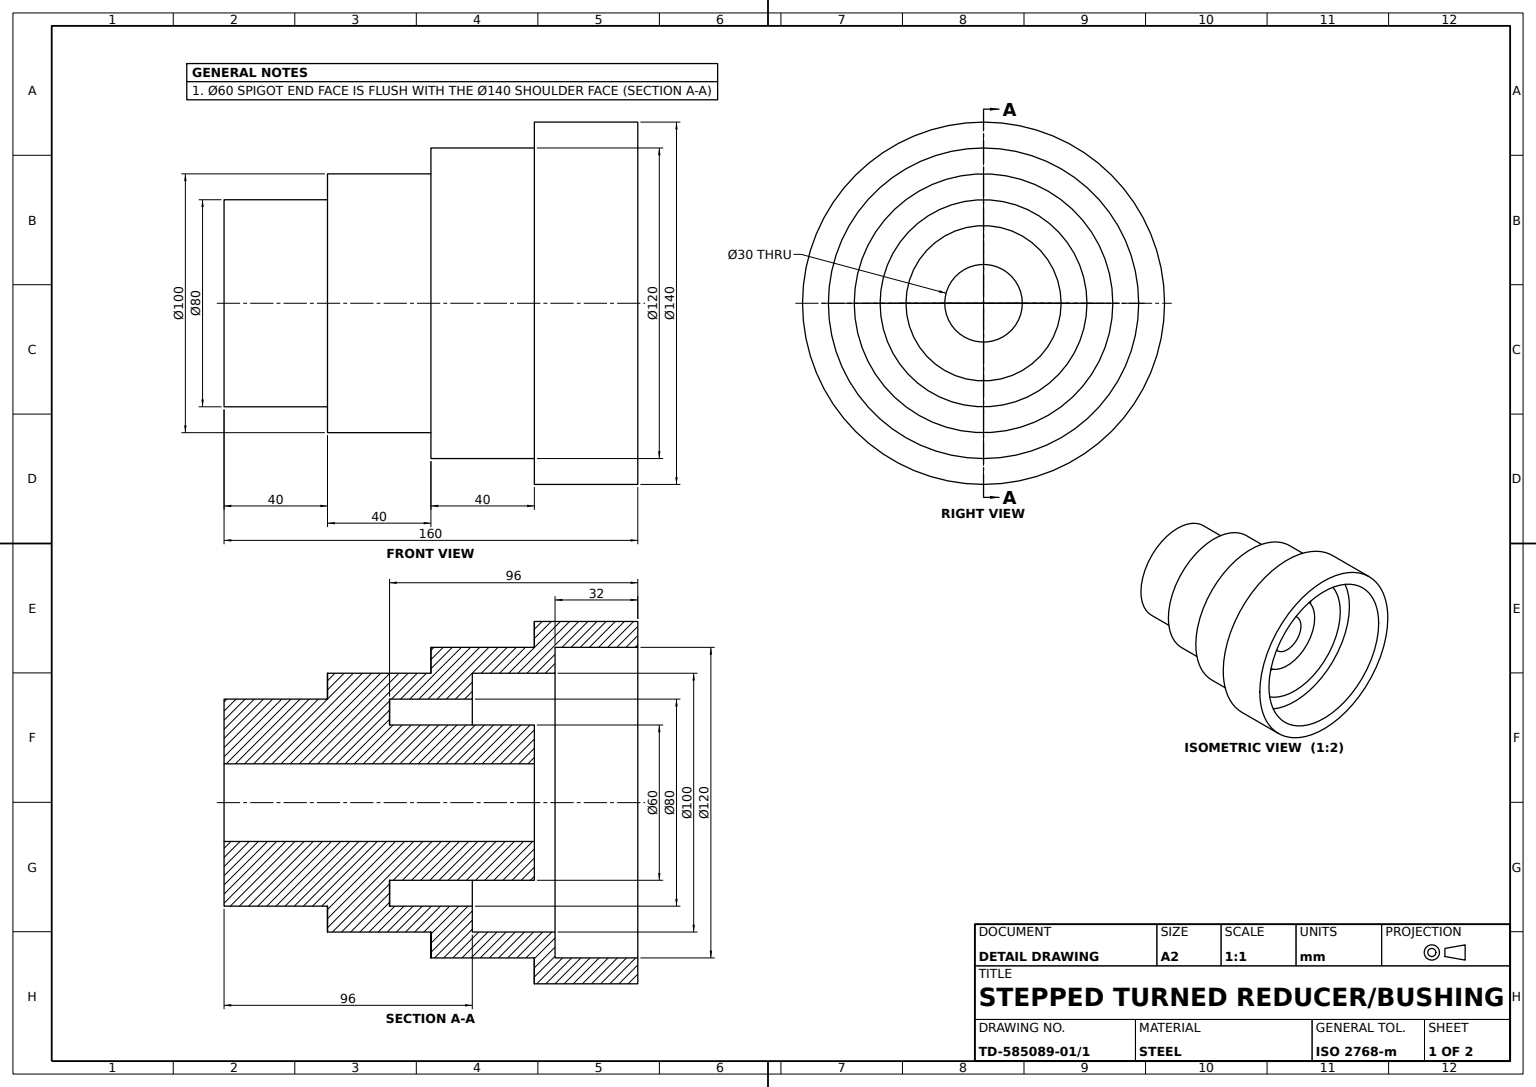
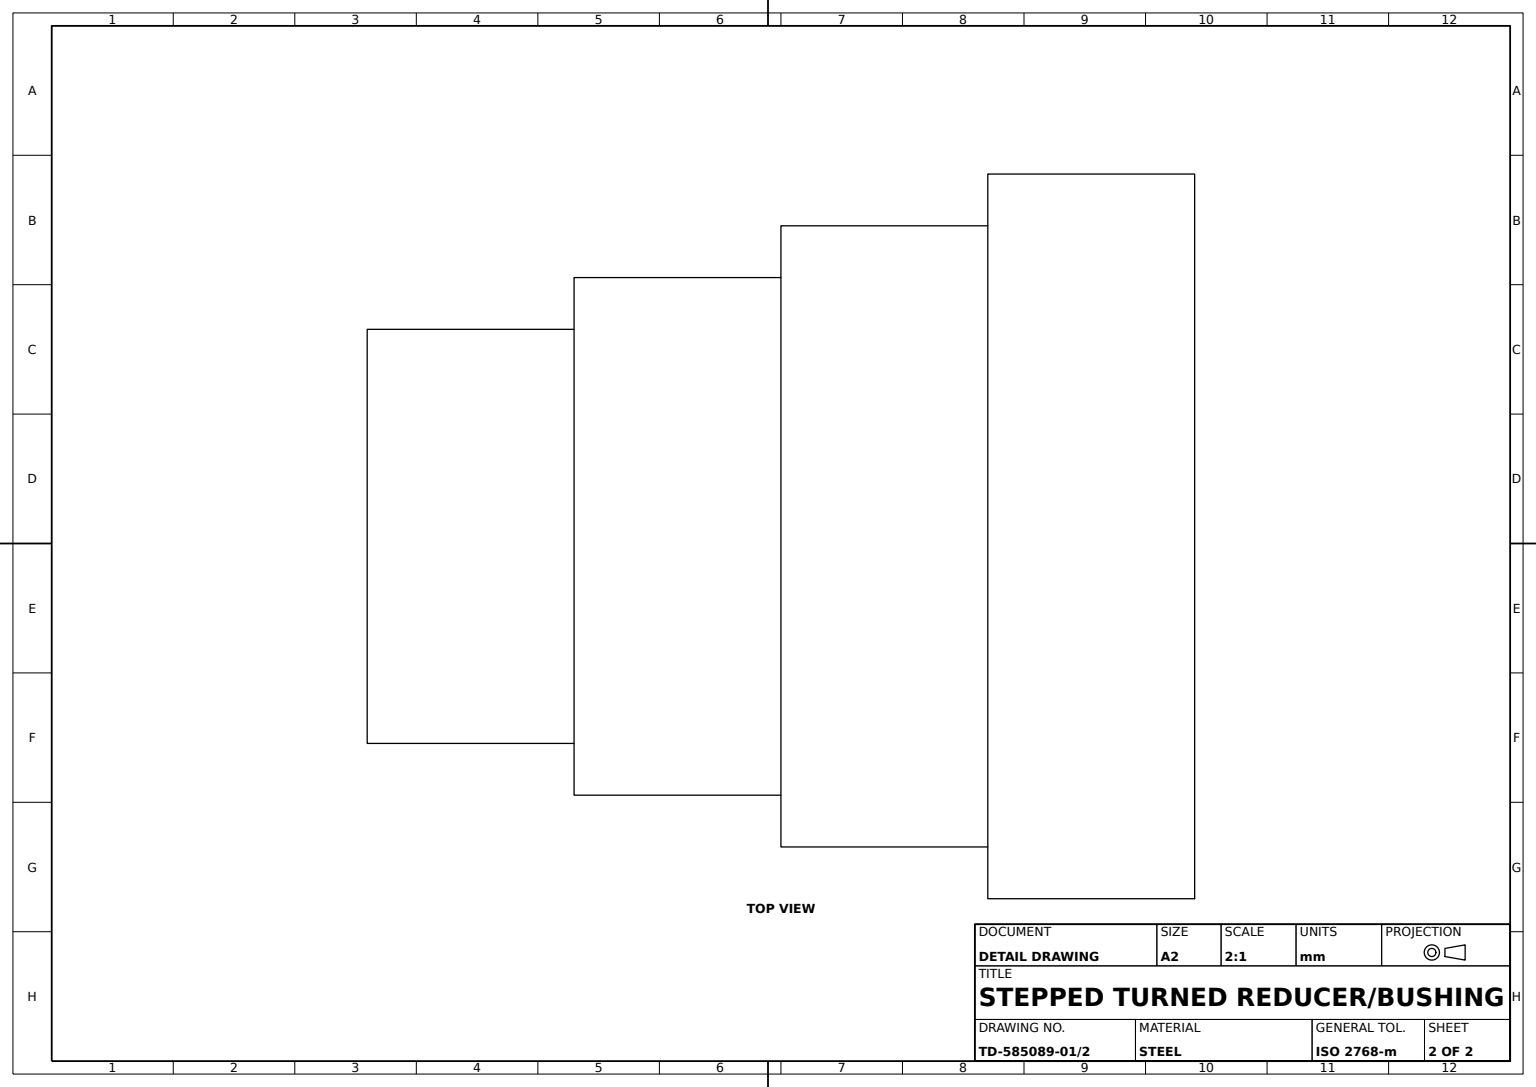
SolidWorks part; units mm, degrees
material "Plain Carbon Steel"
ref_plane "Front Plane" through (0, 0, 0) normal (0, 0, 1) x (1, 0, 0)
ref_plane "Top Plane" through (0, 0, 0) normal (0, 1, 0) x (1, 0, 0)
ref_plane "Right Plane" through (0, 0, 0) normal (1, 0, 0) x (0, 0, -1)
sketch "Stepped Bushing Profile" plane through (0, 0, 0) normal (0, 0, 1) x (1, 0, 0)
  line L0 (-96.9857, 0) -> (110.3939, 0) construction
  line L17 (-42.4079, 15) -> (-42.4079, 40)
  line L18 (-42.4079, 40) -> (-2.4079, 40)
  line L19 (-2.4079, 40) -> (-2.4079, 50)
  line L20 (-2.4079, 50) -> (37.5921, 50)
  line L21 (37.5921, 50) -> (37.5921, 60)
  line L22 (37.5921, 60) -> (77.5921, 60)
  line L23 (77.5921, 60) -> (77.5921, 70)
  line L24 (77.5921, 70) -> (117.5921, 70)
  line L25 (117.5921, 70) -> (117.5921, 60)
  line L26 (117.5921, 60) -> (85.5921, 60)
  line L27 (85.5921, 60) -> (85.5921, 50)
  line L28 (85.5921, 50) -> (53.5921, 50)
  line L29 (53.5921, 50) -> (53.5921, 40)
  line L30 (53.5921, 40) -> (21.5921, 40)
  line L31 (21.5921, 40) -> (21.5921, 30)
  line L32 (-42.4079, 15) -> (77.5921, 15)
  line L33 (77.5921, 15) -> (77.5921, 30)
  line L34 (21.5921, 30) -> (77.5921, 30)
  dimension "D1" = 21.5921
  dimension "D2" = 37.5921
  dimension "D3" = 53.5921
  dimension "D4" = 85.5921
  dimension "D5" = 117.5921
  dimension "D6" = 2.4079
  dimension "D7" = 77.5921
  dimension "D8" = 77.5921
  dimension "D9" = 42.4079
  dimension "D10" = 70
  dimension "D11" = 15
  dimension "D12" = 15
  dimension "D13" = 10
  dimension "D14" = 10
  dimension "D15" = 10
  dimension "D16" = 25
  dimension "D17" = 35
  dimension "D18" = 30
revolve "Stepped Bushing Revolve" add sketch "Stepped Bushing Profile" angle 360 about L0
